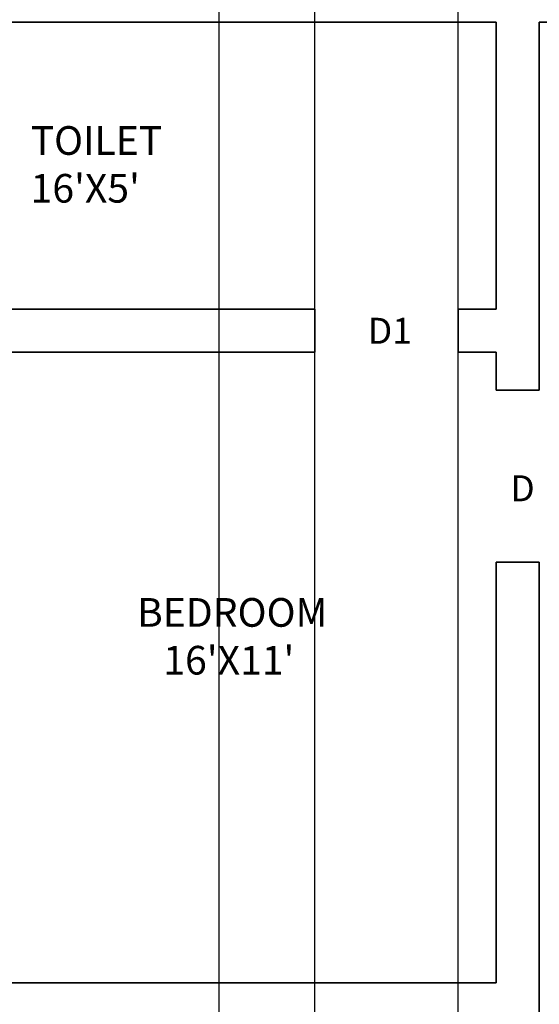
# Model space of a CAD drawing. Units: inches. Extents: x 318 to 927, y -1130 to 13.
# Tile 15 of 17: x 490 to 599, y -297 to -91. Entities that reach past the tile are written whole.
import ezdxf

# ---------------------------------------------------------------- set-up
doc = ezdxf.new("R2010")
doc.units = ezdxf.units.IN
doc.header["$MEASUREMENT"] = 0
for name, color, linetype, lineweight in [('A-ANNO-DIMS', 1, 'Continuous', 18), ('A-ANNO-IDEN', 1, 'Continuous', 13), ('A-AREA-IDEN', 8, 'Continuous', 18), ('wall', 1, 'Continuous', 35)]:
    doc.layers.add(name, color=color, linetype=linetype, lineweight=lineweight)
doc.styles.get("Standard").update_dxf_attribs({"font": 'arial.ttf'})
doc.dimstyles.get("Standard").update_dxf_attribs({"dimtxt": 0.18, "dimasz": 0.18, "dimexe": 0.18, "dimexo": 0.0625, "dimgap": 0.09, "dimtad": 0, "dimtih": 1, "dimtoh": 1, "dimdec": 1, "dimzin": 0, "dimdsep": 46, "dimlunit": 4, "dimtxsty": 'Standard', "dimcen": 0.09, "dimadec": 0, "dimazin": 0, "dimtfac": 1, "dimtdec": 1, "dimtofl": 0, "dimtmove": 0, "dimatfit": 3, "dimfxl": 1, "dimtolj": 1, "dimtzin": 0, "dimarcsym": 0})

# ---------------------------------------------------------------- blocks, each defined once
blk = doc.blocks.new('*D30')
at = {"layer": 'A-ANNO-DIMS', "color": 0, "lineweight": -2, "transparency": 16777216}
for p, q in [((551.89, -820.85), (551.89, -25.23)), ((552.07, -25.41), (566.56, -25.41)), ((581.71, -25.41), (567.23, -25.41)), ((581.89, -820.85), (581.89, -25.23))]:
    blk.add_line(p, q, dxfattribs=at)
at = {"layer": 'A-ANNO-DIMS', "color": 0, "transparency": 16777216}
for points in [[(552.07, -25.38), (552.07, -25.44), (551.89, -25.41)], [(581.71, -25.38), (581.71, -25.44), (581.89, -25.41)]]:
    blk.add_solid(points, dxfattribs=at)
at = {"layer": 'Defpoints', "color": 0, "transparency": 16777216}
for p in [(581.89, -25.41), (551.89, -820.91), (581.89, -820.91)]:
    blk.add_point(p, dxfattribs=at)
at = {"layer": 'A-ANNO-DIMS', "color": 0, "transparency": 16777216, "insert": (566.89, -25.41), "char_height": 0.18, "attachment_point": 5}
blk.add_mtext('\\A1;2\'-6"', dxfattribs=at)
blk = doc.blocks.new('*D33')
at = {"layer": 'A-ANNO-DIMS', "color": 0, "lineweight": -2, "transparency": 16777216}
for p, q in [((397.89, -370.85), (397.89, -25.23)), ((398.07, -25.41), (464.5, -25.41)), ((531.71, -25.41), (465.28, -25.41)), ((531.89, -370.85), (531.89, -25.23))]:
    blk.add_line(p, q, dxfattribs=at)
at = {"layer": 'A-ANNO-DIMS', "color": 0, "transparency": 16777216}
for points in [[(398.07, -25.38), (398.07, -25.44), (397.89, -25.41)], [(531.71, -25.38), (531.71, -25.44), (531.89, -25.41)]]:
    blk.add_solid(points, dxfattribs=at)
at = {"layer": 'Defpoints', "color": 0, "transparency": 16777216}
for p in [(531.89, -25.41), (397.89, -370.91), (531.89, -370.91)]:
    blk.add_point(p, dxfattribs=at)
at = {"layer": 'A-ANNO-DIMS', "color": 0, "transparency": 16777216, "insert": (464.89, -25.41), "char_height": 0.18, "attachment_point": 5}
blk.add_mtext('\\A1;11\'-2"', dxfattribs=at)

msp = doc.modelspace()

# ---------------------------------------------------------------- linework, layer by layer
at = {"layer": 'wall'}
for p, q in [((589.89, -91.91), (397.89, -91.91)), ((589.89, -91.91), (589.89, -151.91)), ((598.89, -91.91), (598.89, -168.91)), ((718.89, -91.91), (598.89, -91.91)), ((551.89, -151.91), (397.89, -151.91)), ((551.89, -151.91), (551.89, -160.91)), ((589.89, -151.91), (581.89, -151.91)), ((581.89, -151.91), (581.89, -160.91)), ((551.89, -160.91), (397.89, -160.91)), ((589.89, -160.91), (581.89, -160.91)), ((589.89, -160.91), (589.89, -168.91)), ((598.89, -168.91), (589.89, -168.91)), ((598.89, -204.91), (589.89, -204.91)), ((589.89, -204.91), (589.89, -292.91)), ((598.89, -204.91), (598.89, -309.91)), ((589.89, -292.91), (397.89, -292.91)), ((589.89, -292.91), (397.89, -292.91))]:
    msp.add_line(p, q, dxfattribs=at)

# ---------------------------------------------------------------- texts
at = {"layer": 'A-ANNO-IDEN'}
for s, height, p in [('D1', 5.444, (563, -159.19)), ('D', 5.44, (592.83, -192.15))]:
    msp.add_text(s, height=height, dxfattribs=at).set_placement(p)
at = {"layer": 'A-AREA-IDEN', "char_height": 6, "attachment_point": 1}
for s, width, insert in [("       TOILET\\P       16'X5'", 54.3765, (479.6, -113.64)), (" BEDROOM\\P    16'X11'", 45.6749, (512.88, -212.4))]:
    msp.add_mtext_dynamic_manual_height_columns(s, width=width, gutter_width=1, heights=[0], dxfattribs=dict(at, insert=insert))

# ---------------------------------------------------------------- dimensions: what is measured, and where the dimension line sits
at = {"layer": 'A-ANNO-DIMS'}
for base, p1, p2, picture, middle in [((531.89, -25.41), (397.89, -370.91), (531.89, -370.91), '*D33', (464.89, -25.41)), ((581.89, -25.41), (551.89, -820.91), (581.89, -820.91), '*D30', (566.89, -25.41))]:
    dim = msp.add_linear_dim(base=base, p1=p1, p2=p2, dimstyle='Standard', override={"dimdec": 1, "dimlfac": 1, "dimrnd": 0, "dimzin": 1, "dimdsep": 46, "dimlunit": 4, "dimfrac": 2}, dxfattribs=at)
    dim.commit()
    dim.dimension.update_dxf_attribs({"geometry": picture, "text_midpoint": middle})

doc.saveas('drawing.dxf')
